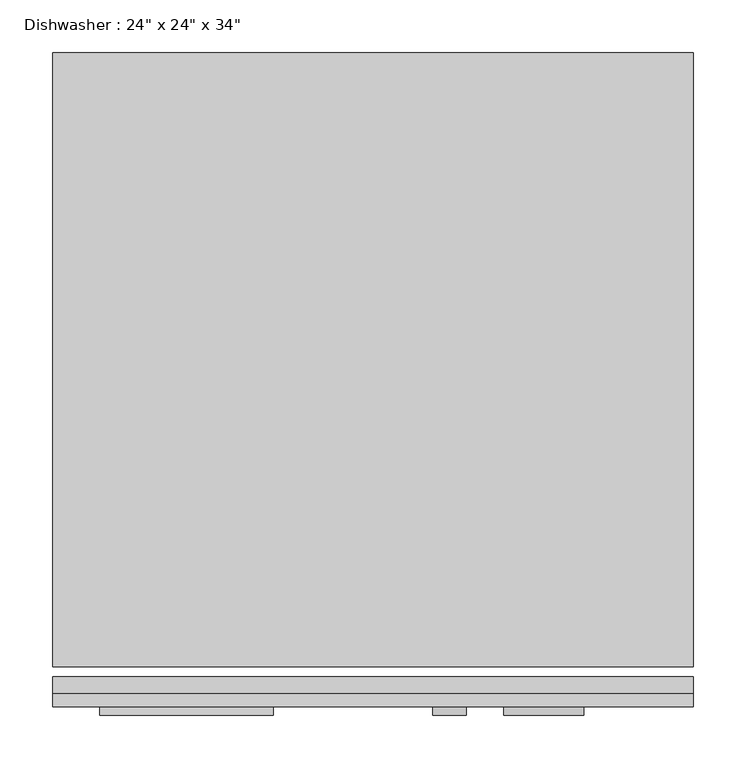
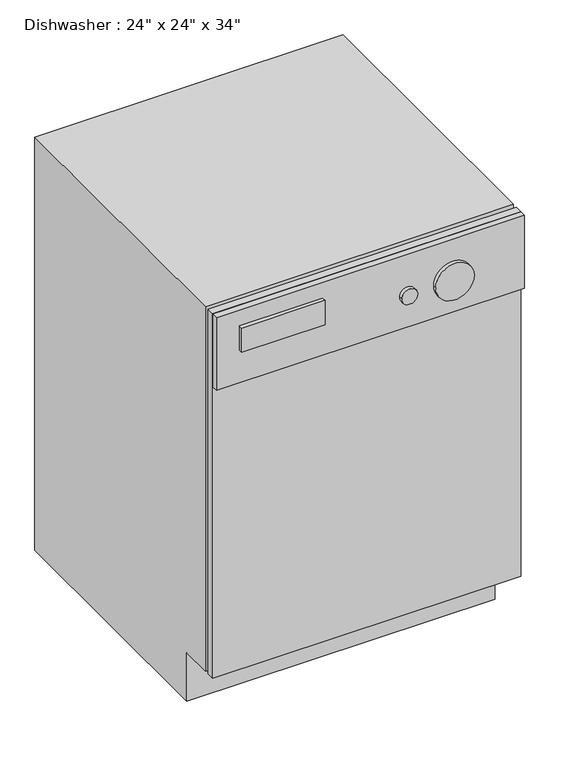
"""IFC4 building model written with IfcOpenShell, lengths in millimetres: proxy geometry."""

from ifc_helpers import new_model, si_unit, point, frame, frame_2d, origin, place, context, project, spatial, polyline, circle_curve, trimmed, segment, composite_curve, outline, extrude, source, transform, mapped, element, save


def proxy_45b28599(model_context):
    return source(origin(), model_context, "Body", "SweptSolid", [
        extrude(outline(polyline([(687.1174685, -38.3504352), (77.5174685, -38.3504352), (77.5174685, -22.4754352), (687.1174685, -22.4754352), (687.1174685, -38.3504352)])), frame((0.0, 0.0, 101.6), z_axis=(0.0, 0.0, 1.0), x_axis=(1.0, 0.0, 0.0)), (0.0, 0.0, 1.0), 762.0),
        extrude(outline(polyline([(687.1174685, -38.3504352), (687.1174685, -51.0504352), (77.5174685, -51.0504352), (77.5174685, -38.3504352), (687.1174685, -38.3504352)])), frame((0.0, 0.0, 711.2), z_axis=(0.0, 0.0, 1.0), x_axis=(1.0, 0.0, 0.0)), (0.0, 0.0, 1.0), 152.4),
        extrude(outline(polyline([(571.2495648, 0.0), (50.5495648, 0.0), (50.5495648, 101.6), (-12.9504352, 101.6), (-12.9504352, 863.6), (571.2495648, 863.6), (571.2495648, 0.0)])), frame((77.5174685, 0.0, 0.0), z_axis=(1.0, 0.0, 0.0), x_axis=(0.0, 1.0, 0.0)), (0.0, 0.0, 1.0), 609.6),
        extrude(outline(polyline([(287.6378068, -59.1863727), (122.5378068, -59.1863727), (122.5378068, -51.0504352), (287.6378068, -51.0504352), (287.6378068, -59.1863727)])), frame((0.0, 0.0, 780.0846419), z_axis=(0.0, 0.0, 1.0), x_axis=(1.0, 0.0, 0.0)), (0.0, 0.0, 1.0), 50.8),
        extrude(outline(composite_curve([segment(trimmed(circle_curve(frame_2d((780.0846419, 544.7247133)), 38.1), [point((780.0846419, 506.6247133))], [point((780.0846419, 582.8247133))], False, "CARTESIAN"), True, "CONTINUOUS"), segment(trimmed(circle_curve(frame_2d((780.0846419, 544.7247133)), 38.1), [point((780.0846419, 582.8247133))], [point((780.0846419, 506.6247133))], False, "CARTESIAN"), True, "CONTINUOUS")], self_intersect=False)), frame((0.0, -59.1863727, 0.0), z_axis=(0.0, 1.0, 0.0), x_axis=(0.0, 0.0, 1.0)), (0.0, 0.0, 1.0), 8.1359375),
        extrude(outline(composite_curve([segment(trimmed(circle_curve(frame_2d((780.0846419, 455.195318)), 15.875), [point((780.0846419, 439.320318))], [point((780.0846419, 471.070318))], False, "CARTESIAN"), True, "CONTINUOUS"), segment(trimmed(circle_curve(frame_2d((780.0846419, 455.195318)), 15.875), [point((780.0846419, 471.070318))], [point((780.0846419, 439.320318))], False, "CARTESIAN"), True, "CONTINUOUS")], self_intersect=False)), frame((0.0, -59.1863727, 0.0), z_axis=(0.0, 1.0, 0.0), x_axis=(0.0, 0.0, 1.0)), (0.0, 0.0, 1.0), 8.1359375),
    ])


if __name__ == "__main__":
    model = new_model("IFC4")
    model_context = context("Model", 3, world=origin())
    ifc_project = project(units=[si_unit("LENGTHUNIT", "METRE", prefix="MILLI")], contexts=[model_context])
    site = spatial("IfcSite", under=ifc_project)
    building = spatial("IfcBuilding", under=site)
    placement = place(None, origin())
    proxy_shape = proxy_45b28599(model_context)
    element("IfcBuildingElementProxy", 1, Name="Dishwasher : 24\" x 24\" x 34\"", ObjectType="Dishwasher : 24\" x 24\" x 34\"", at=placement, inside=building, context=model_context, shape_type="MappedRepresentation", body=[
        mapped(proxy_shape, transform((0.0, 0.0, 0.0), x_axis=(1.0, 0.0, 0.0), y_axis=(0.0, 1.0, 0.0), z_axis=(0.0, 0.0, 1.0))),
    ])
    save(model, "model.ifc")

# Revit data of these elements
# Type "Dishwasher : 24\" x 24\" x 34\""
#   Label = "DW"
#   Assembly Code = "E1090400"
#   Depth = 2' - 0"
#   Height = 2' - 10"
#   Width = 2' - 0"
#   Dishwasher Material = Steel, Paint Finish, Ivory, Glossy
#   Panel Face Material = Plastic, Opaque Black
#   Default Elevation = 0
# Element 1 (IfcBuildingElementProxy, "Dishwasher : 24\" x 24\" x 34\"")
#   Materials on its faces: "Steel, Paint Finish, Ivory, Glossy", "Plastic, Opaque Black"
# Materials
#   "Steel, Paint Finish, Ivory, Glossy": class "Metal", colour RGB 247 247 239, transparency 0, Description = "Steel, paint finish, ivory, glossy", Cost = 0
#   "Plastic, Opaque Black": class "Plastic", colour RGB 0 0 0, transparency 0.05, Description = "Plastic, generic, opaque black", Cost = 0
